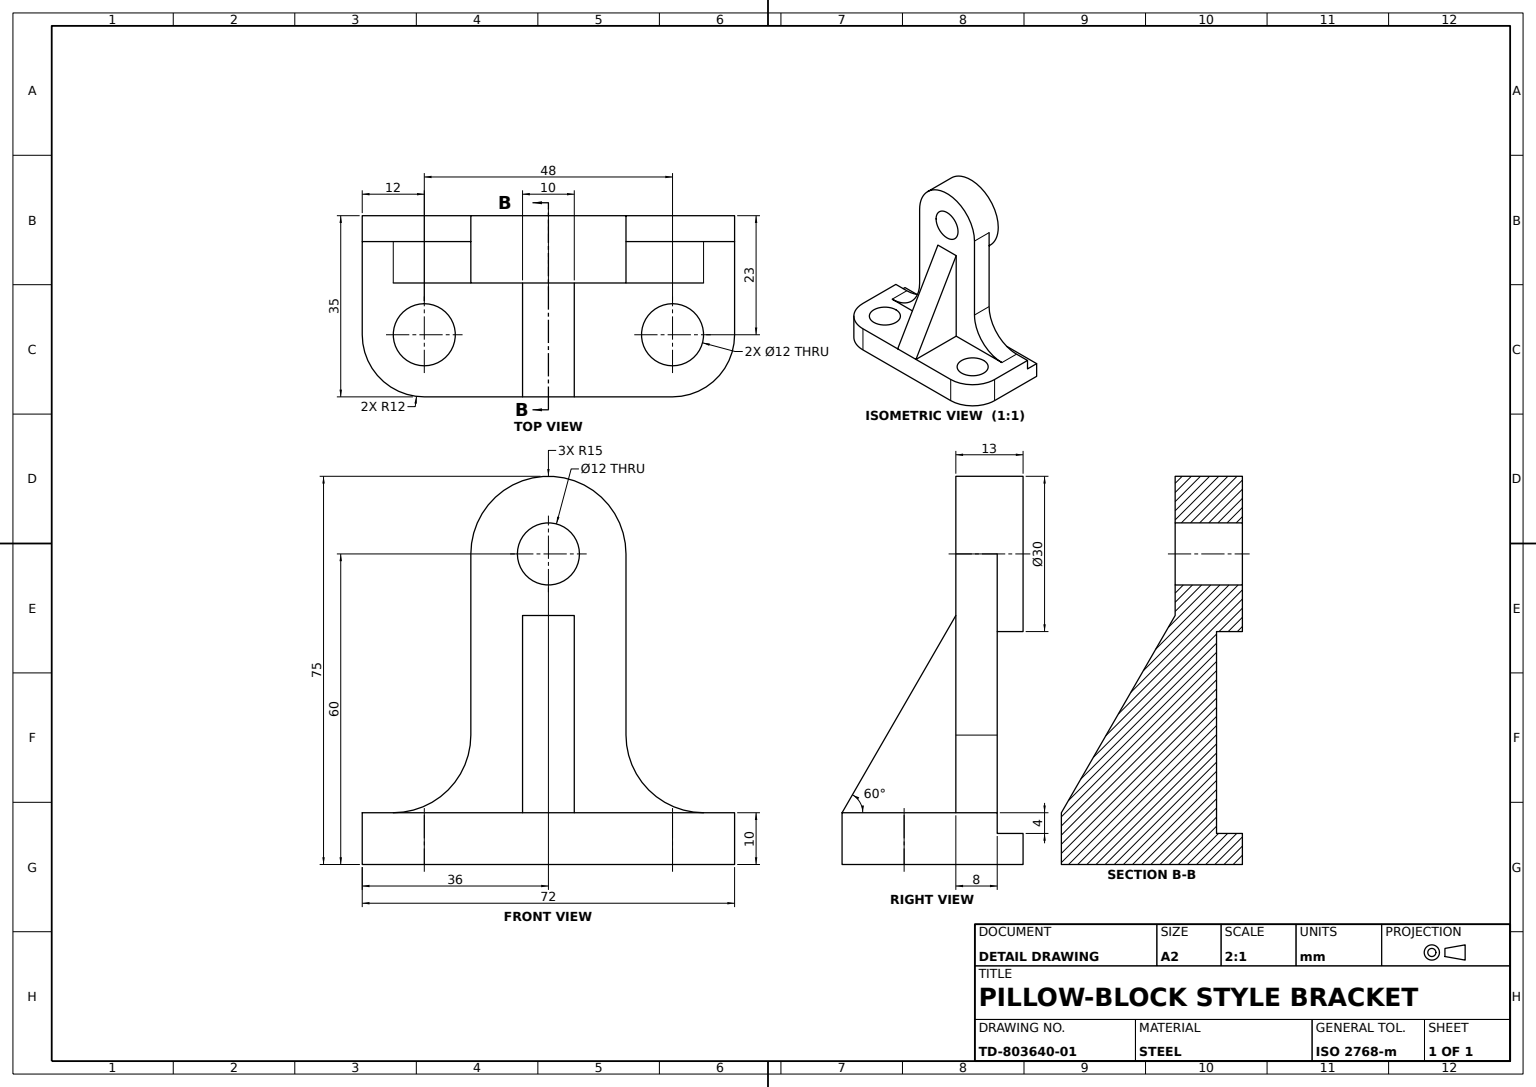
from build123d import *

# Parameters (mm, degrees)
BASE_PLATE_SKETCH_R       = 6
BASE_PLATE_DEPTH          = 10
REAR_GROOVE_SKETCH_W      = 5
REAR_GROOVE_SKETCH_H      = 4
REAR_GROOVE_4X5_DEPTH     = 77.243032469
UPRIGHT_SKETCH_W          = 30
UPRIGHT_SKETCH_H          = 50
UPRIGHT_DEPTH             = 8
HUB_BOSS_SKETCH_R         = 15
HUB_BOSS_SKETCH_R_2       = 6
HUB_BOSS_DEPTH            = 13
SHAFT_START               = -13
SHAFT_BORE_SKETCH_R       = 6
SHAFT_BORE_DEPTH          = 13
UPRIGHT_BASE_FILLET_R15_R = 15
SUPPORT_RIB_REACH         = 88.313
SUPPORT_RIB_SKETCH_WALL_W = 218.626765016
SUPPORT_RIB_SKETCH_WALL_H = 10


with BuildPart() as part:
    # Base Plate Sketch → Base Plate (new body)
    with BuildSketch(Plane(origin=(0, 0, 0), x_dir=(1, 0, 0), z_dir=(0, 1, 0))):
        with BuildLine():
            Line((-36, 23), (-36, 0))
            ThreePointArc((-36, 0), (-32.485281374, -8.485281374), (-24, -12))
            Line((-24, -12), (24, -12))
            ThreePointArc((24, -12), (32.485281374, -8.485281374), (36, 0))
            Line((36, 0), (36, 23))
            Line((36, 23), (-36, 23))
        make_face()
        with Locations(Location((-24, 0, 0), (0, 0, 270))):
            Circle(BASE_PLATE_SKETCH_R, mode=Mode.SUBTRACT)
        with Locations(Location((24, 0, 0), (0, 0, 90))):
            Circle(BASE_PLATE_SKETCH_R, mode=Mode.SUBTRACT)
    extrude(amount=BASE_PLATE_DEPTH)

    # Rear Groove Sketch → Rear Groove 4x5 (cut, through all)
    with BuildSketch(Plane(origin=(36, 0, 0), x_dir=(0, 0, -1), z_dir=(1, 0, 0))):
        with Locations((20.5, 8)):
            Rectangle(REAR_GROOVE_SKETCH_W, REAR_GROOVE_SKETCH_H)
    extrude(amount=-REAR_GROOVE_4X5_DEPTH, mode=Mode.SUBTRACT)

    # Upright Sketch → Upright (add)
    with BuildSketch(Plane.XY.offset(-18)):
        with Locations((0, 35)):
            Rectangle(UPRIGHT_SKETCH_W, UPRIGHT_SKETCH_H)
    extrude(amount=UPRIGHT_DEPTH)

    # Hub Boss Sketch → Hub Boss (add)
    with BuildSketch(Plane.XY.offset(-10)):
        with Locations((0, 60)):
            Circle(HUB_BOSS_SKETCH_R)
        with Locations((0, 60)):
            Circle(HUB_BOSS_SKETCH_R_2, mode=Mode.SUBTRACT)
    extrude(amount=-HUB_BOSS_DEPTH)

    # Shaft Bore Sketch → Shaft Bore (cut)
    with BuildSketch(Plane(origin=(0, 0, -23), x_dir=(-1, 0, 0), z_dir=(0, 0, -1)).offset(SHAFT_START)):
        with Locations(Location((0, 60, 0), (0, 0, 180))):
            Circle(SHAFT_BORE_SKETCH_R)
    extrude(amount=SHAFT_BORE_DEPTH, mode=Mode.SUBTRACT)

    # Upright Base Fillet R15
    upright_base_fillet_r15_edges = [part.edges().sort_by_distance(p)[0] for p in [
        (-15, 10, -14),
        (15, 10, -14),
    ]]
    fillet(upright_base_fillet_r15_edges, radius=UPRIGHT_BASE_FILLET_R15_R)

    # Support Rib Sketch wall → Support Rib (add, up to next)
    with BuildSketch(Plane(origin=(0, 29.052558884, 1), x_dir=(0, 0.866025403787, -0.499999999995), z_dir=(0, 0.499999999995, 0.866025403787)), mode=Mode.PRIVATE) as support_rib_sk1:
        Rectangle(SUPPORT_RIB_SKETCH_WALL_W, SUPPORT_RIB_SKETCH_WALL_H)
    support_rib_tool1 = extrude(support_rib_sk1.sketch, amount=-SUPPORT_RIB_REACH, mode=Mode.PRIVATE) - part.part
    add(support_rib_tool1.solids().sort_by_distance((0, 29.052558884, 1))[0])


solid = part.part
